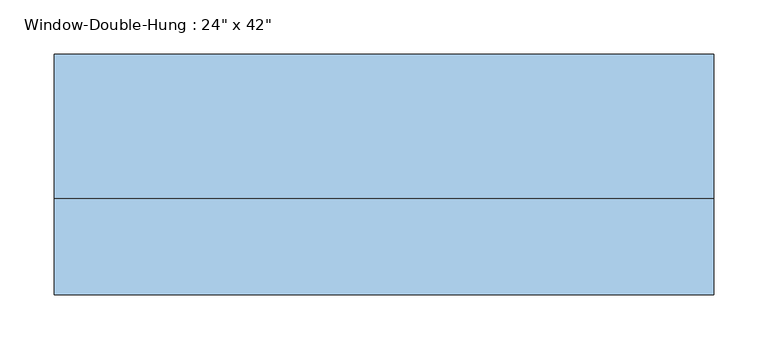
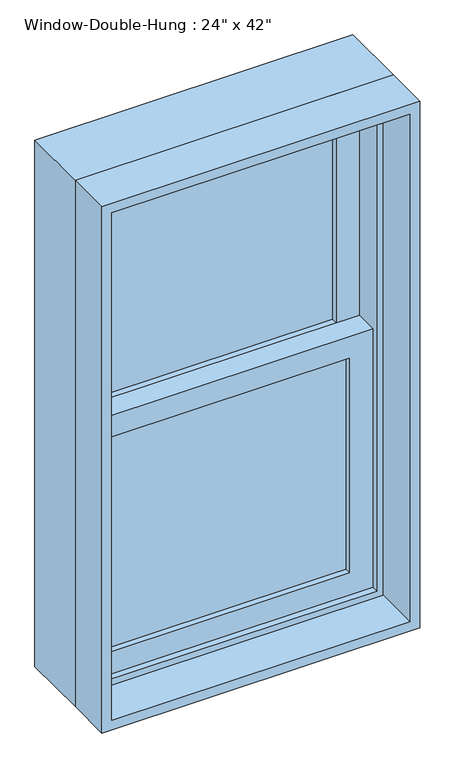
"""IFC4 building model written with IfcOpenShell, lengths in millimetres: window geometry."""

from ifc_helpers import new_model, si_unit, frame, origin, place, context, project, spatial, polyline, outline, extrude, source, transform, mapped, element, save


def window_679d2811(model_context):
    return source(origin(), model_context, "Body", "SweptSolid", [
        extrude(outline(polyline([(228.6, 31.75), (228.6, 25.4), (-228.6, 25.4), (-228.6, 31.75), (228.6, 31.75)])), frame((0.0, 0.0, 990.6), z_axis=(0.0, 0.0, 1.0), x_axis=(1.0, 0.0, 0.0)), (0.0, 0.0, 1.0), 434.975),
        extrude(outline(polyline([(-228.6, 19.05), (228.6, 19.05), (228.6, 12.7), (-228.6, 12.7), (-228.6, 19.05)])), frame((0.0, 0.0, 990.6), z_axis=(0.0, 0.0, 1.0), x_axis=(1.0, 0.0, 0.0)), (0.0, 0.0, 1.0), 434.975),
        extrude(outline(polyline([(228.6, 76.2), (228.6, 69.85), (-228.6, 69.85), (-228.6, 76.2), (228.6, 76.2)])), frame((0.0, 0.0, 1470.025), z_axis=(0.0, 0.0, 1.0), x_axis=(1.0, 0.0, 0.0)), (0.0, 0.0, 1.0), 434.975),
        extrude(outline(polyline([(-228.6, 63.5), (228.6, 63.5), (228.6, 57.15), (-228.6, 57.15), (-228.6, 63.5)])), frame((0.0, 0.0, 1470.025), z_axis=(0.0, 0.0, 1.0), x_axis=(1.0, 0.0, 0.0)), (0.0, 0.0, 1.0), 434.975),
        extrude(outline(polyline([(1470.025, -273.05), (946.15, -273.05), (946.15, 273.05), (1470.025, 273.05), (1470.025, -273.05)]), holes=[polyline([(1425.575, 228.6), (990.6, 228.6), (990.6, -228.6), (1425.575, -228.6), (1425.575, 228.6)])]), frame((0.0, 0.0, 0.0), z_axis=(0.0, 1.0, 0.0), x_axis=(0.0, 0.0, 1.0)), (0.0, 0.0, 1.0), 44.45),
        extrude(outline(polyline([(1949.45, -273.05), (1425.575, -273.05), (1425.575, 273.05), (1949.45, 273.05), (1949.45, -273.05)]), holes=[polyline([(1905.0, 228.6), (1470.025, 228.6), (1470.025, -228.6), (1905.0, -228.6), (1905.0, 228.6)])]), frame((0.0, 44.45, 0.0), z_axis=(0.0, 1.0, 0.0), x_axis=(0.0, 0.0, 1.0)), (0.0, 0.0, 1.0), 44.45),
        extrude(outline(polyline([(1981.2, -304.8), (914.4, -304.8), (914.4, 304.8), (1981.2, 304.8), (1981.2, -304.8)]), holes=[polyline([(1949.45, 273.05), (946.15, 273.05), (946.15, -273.05), (1949.45, -273.05), (1949.45, 273.05)])]), frame((0.0, -12.7, 0.0), z_axis=(0.0, 1.0, 0.0), x_axis=(0.0, 0.0, 1.0)), (0.0, 0.0, 1.0), 133.35),
        extrude(outline(polyline([(1981.2, 304.8), (1981.2, -304.8), (914.4, -304.8), (914.4, 304.8), (1981.2, 304.8)]), holes=[polyline([(1962.15, 285.75), (933.45, 285.75), (933.45, -285.75), (1962.15, -285.75), (1962.15, 285.75)])]), frame((0.0, -101.6, 0.0), z_axis=(0.0, 1.0, 0.0), x_axis=(0.0, 0.0, 1.0)), (0.0, 0.0, 1.0), 88.9),
    ])


if __name__ == "__main__":
    model = new_model("IFC4")
    model_context = context("Model", 3, world=origin())
    ifc_project = project(units=[si_unit("LENGTHUNIT", "METRE", prefix="MILLI")], contexts=[model_context])
    site = spatial("IfcSite", under=ifc_project)
    building = spatial("IfcBuilding", under=site)
    placement = place(None, origin())
    window_shape = window_679d2811(model_context)
    element("IfcWindow", 1, ObjectType="Window-Double-Hung : 24\" x 42\"", at=placement, inside=building, context=model_context, shape_type="MappedRepresentation", body=[
        mapped(window_shape, transform((0.0, 0.0, 0.0), x_axis=(1.0, 0.0, 0.0), y_axis=(0.0, 1.0, 0.0), z_axis=(0.0, 0.0, 1.0))),
    ])
    save(model, "model.ifc")

# Revit data of these elements
# Type "Window-Double-Hung : 24\" x 42\""
#   Type Mark = "10"
#   Fire Rating = "0.5h"
#   Construction Type Id = "DG-DR"
#   Assembly Code = "B2020100"
#   Analytic Construction = "Double glazing - domestic"
#   Wall Thickness [instance default] = 0' - 6"
#   Window Inset [instance default] = 0' - 0"
#   Visual Light Transmittance = 0.81
#   Thermal Resistance (R) = 1.8146 (h·ft²·°F)/BTU
#   Solar Heat Gain Coefficient = 0.76
#   Muntin Width = 1' - 6"
#   Muntin Height = 1' - 5 1/8"
#   Interior Wall Closure [instance default] = 0' - 1 1/2"
#   Rough Width = 2' - 0 1/2"
#   Rough Height = 3' - 6 1/2"
#   Frame Extension [instance default] = 0' - 1 1/4"
#   Exterior Wall Closure [instance default] = 0' - 0 1/2"
#   Extension Jamb [instance default] = 0' - 1 1/2"
#   Heat Transfer Coefficient (U) = 0.5511 BTU/(h·ft²·°F)
#   Height = 3' - 6"
#   Width = 2' - 0"
#   Define Thermal Properties by = 1
#   Top Muntin Visibility = yes
#   Indicator Visibility [instance default] = yes
#   Extension Jamb Visibility [instance default] = yes
#   Interior Trim Visibility [instance default] = yes
#   Exterior Trim Visibility [instance default] = yes
#   Define Thermal Properties by = 1
#   Bottom Muntin Visibility = yes
#   Muntin Pattern = Muntin Pattern_2x2 : Muntin Pattern_2x2
#   Interior Trim Material = Wood - Stained
#   Interior Trim = Trim-Window-Interior-Flat : Picture Frame
#   Exterior Trim Material = Clad - White
#   Exterior Trim = Trim-Window-Exterior-Flat : with Sill
#   Glass Panel Material = Glass
#   Exterior Frame Material = Clad - White
#   Interior Frame Material = Wood - Stained
#   Wall Closure = (empty or 0)
# Element 1 (IfcWindow, "Window-Double-Hung : 24\" x 42\"")
#   Wall Thickness = 0' - 8"
#   Extension Jamb = 0' - 3 1/2"
#   Materials on its faces: "Wood - Stained", "Glass", "Clad - White"
# Materials
#   "Wood - Stained": class "Wood", colour RGB 224 178 126, transparency 0, Cost = 0
#   "Clad - White": class "Wood", colour RGB 242 242 238, transparency 0, Cost = 0
#   "Glass": class "Glass", colour RGB 0 128 192, transparency 0.75, Description = "Soda Lime Glass", Cost = 0
